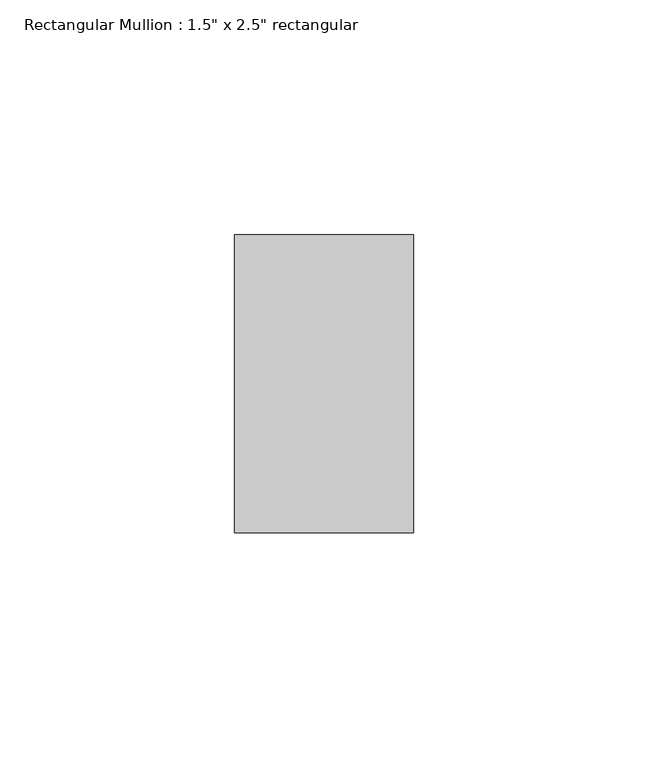
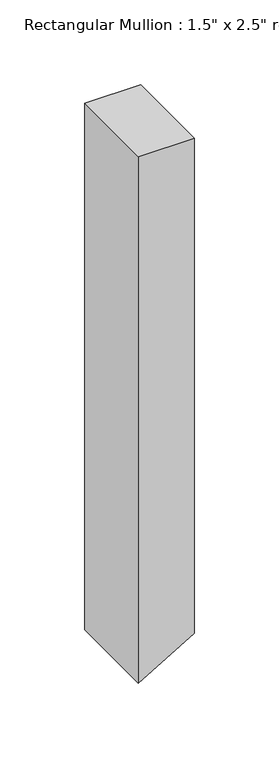
"""IFC4 building model written with IfcOpenShell, lengths in millimetres: member geometry."""

from ifc_helpers import new_model, si_unit, frame, origin, place, context, project, spatial, polyline, outline, extrude, source, transform, mapped, element, save


def member_c8c782b1(model_context):
    return source(origin(), model_context, "Body", "SweptSolid", [
        extrude(outline(polyline([(0.0, 19.05), (0.0, -19.05), (-379.6932431, -19.05), (-357.0487292, 19.05), (0.0, 19.05)])), frame((0.0, -31.75, 0.0), z_axis=(0.0, 1.0, 0.0), x_axis=(0.0, 0.0, 1.0)), (0.0, 0.0, 1.0), 63.5),
    ])


if __name__ == "__main__":
    model = new_model("IFC4")
    model_context = context("Model", 3, world=origin())
    ifc_project = project(units=[si_unit("LENGTHUNIT", "METRE", prefix="MILLI")], contexts=[model_context])
    site = spatial("IfcSite", under=ifc_project)
    building = spatial("IfcBuilding", under=site)
    placement = place(None, origin())
    member_shape = member_c8c782b1(model_context)
    element("IfcMember", 1, ObjectType="Rectangular Mullion : 1.5\" x 2.5\" rectangular", at=placement, inside=building, context=model_context, shape_type="MappedRepresentation", body=[
        mapped(member_shape, transform((0.0, 0.0, 0.0), x_axis=(1.0, 0.0, 0.0), y_axis=(0.0, 1.0, 0.0), z_axis=(0.0, 0.0, 1.0))),
    ])
    save(model, "model.ifc")

# Revit data of these elements
# Type "Rectangular Mullion : 1.5\" x 2.5\" rectangular"
#   built-in parameter 1007304 = 0.208333 (stored number, unit not read)
#   built-in parameter 1007301 = 0.0625 (stored number, unit not read)
#   built-in parameter 1007300 = 0.0625 (stored number, unit not read)
